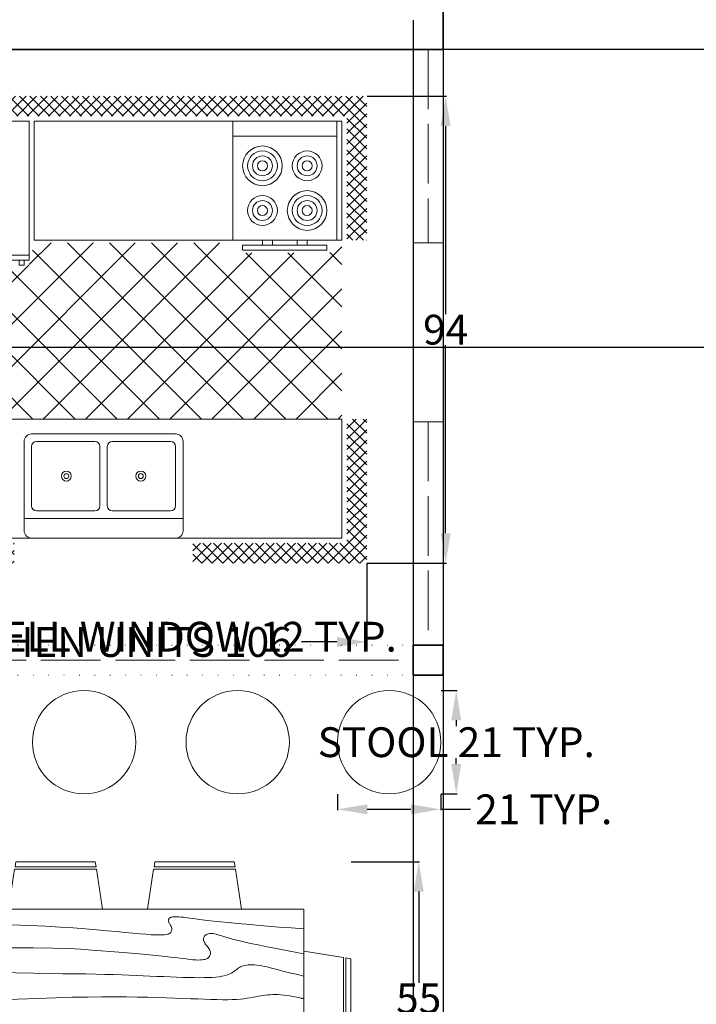
# Model space of a CAD drawing. Units: inches. Extents: x 823 to 1335, y 207 to 1074.
# Tile 4 of 6: x 943 to 1079, y 577 to 776. Entities that reach past the tile are written whole.
import ezdxf

# ---------------------------------------------------------------- set-up
doc = ezdxf.new("R2010")
doc.units = ezdxf.units.IN
doc.header["$MEASUREMENT"] = 0
doc.linetypes.add('ACAD_ISO02W100', pattern=[15, 12, -3])
doc.linetypes.add('ACAD_ISO07W100', pattern=[3, 0, -3])
for name, color, linetype, lineweight in [('A-ANNO-DIMS', 2, 'Continuous', 18), ('A-GLAZ-HIDN', 211, 'ACAD_ISO02W100', 18), ('A-GLAZ-OVHD', 211, 'ACAD_ISO07W100', 18), ('furniture', 21, 'Continuous', 18), ('inner wall', 102, 'Continuous', 35), ('kitchen', 171, 'Continuous', 18), ('windows', 211, 'Continuous', 18)]:
    doc.layers.add(name, color=color, linetype=linetype, lineweight=lineweight)
doc.styles.get("Standard").update_dxf_attribs({"font": 'arial.ttf'})
doc.dimstyles.get("Standard").update_dxf_attribs({"dimtxt": 6, "dimasz": 6, "dimexe": 0.18, "dimexo": 0.0625, "dimgap": 0.09, "dimtad": 0, "dimtih": 1, "dimtoh": 1, "dimdec": 0, "dimzin": 0, "dimdsep": 46, "dimlunit": 3, "dimtxsty": 'Standard', "dimcen": 0.09, "dimadec": 0, "dimazin": 0, "dimtfac": 1, "dimtdec": 0, "dimtofl": 0, "dimtmove": 0, "dimatfit": 3, "dimfxl": 1, "dimtolj": 1, "dimtzin": 0, "dimarcsym": 0})

# ---------------------------------------------------------------- blocks, each defined once
blk = doc.blocks.new('Dining Set - 36 x 72 in.')
for p, q in [((-22.2343, 26.00059), (-23.4847, 17.99762)), ((-22.2304, 26), (-5.7608, 26)), ((-22, 27.5), (-22.1562, 26.50042)), ((-5.8416, 26.5), (-22.1534, 26.5)), ((-22, 27.5), (-6, 27.5)), ((-5.8437, 26.49966), (-6, 27.5)), ((-4.5152, 17.99762), (-5.7655, 25.99926)), ((5.7657, 26.00059), (4.5153, 17.99762)), ((5.7696, 26), (22.2392, 26)), ((6, 27.5), (5.8438, 26.50042)), ((22.1584, 26.5), (5.8466, 26.5)), ((6, 27.5), (22, 27.5)), ((22.1563, 26.49966), (22, 27.5)), ((23.4848, 17.99762), (22.2345, 25.99926)), ((36, 18), (-36, 18)), ((-36, 18), (-36, -18)), ((36, -18), (36, 18)), ((-45.5, 8), (-44.5004, 8.15617)), ((-45.5, 8), (-45.5, -8)), ((-44.5, -8.15843), (-44.5, 8.15338)), ((-44.0006, 8.23428), (-35.9976, 9.48474)), ((-44, 8.23041), (-44, -8.23915)), ((44.0006, 8.23428), (35.9976, 9.48474)), ((44, 8.23041), (44, -8.23915)), ((44.5, -8.15843), (44.5, 8.15338)), ((45.5, 8), (44.5005, 8.15617)), ((45.5, 8), (45.5, -8)), ((-44.4997, -8.15631), (-45.5, -8)), ((-35.9976, -9.48476), (-43.9993, -8.2345)), ((35.9976, -9.48476), (43.9993, -8.2345)), ((44.4997, -8.15631), (45.5, -8)), ((-36, -18), (36, -18)), ((-22.2343, -26.0006), (-23.4847, -17.99762)), ((-4.5152, -17.99762), (-5.7655, -25.99928)), ((5.7657, -26.0006), (4.5153, -17.99762)), ((23.4848, -17.99762), (22.2345, -25.99928)), ((-22.2304, -26), (-5.7608, -26)), ((-22, -27.5), (-22.1562, -26.50044)), ((-5.8416, -26.5), (-22.1534, -26.5)), ((-22, -27.5), (-6, -27.5)), ((-5.8437, -26.49967), (-6, -27.5)), ((5.7696, -26), (22.2392, -26)), ((6, -27.5), (5.8438, -26.50044)), ((22.1584, -26.5), (5.8466, -26.5)), ((6, -27.5), (22, -27.5)), ((22.1563, -26.49967), (22, -27.5))]:
    blk.add_line(p, q)
for points in [[(-36, 15), (-31.1772, 14.97754), (-26.8079, 14.91406), (-22.8538, 14.81543), (-19.276, 14.6875), (-16.0362, 14.53613), (-13.0957, 14.36718), (-10.4159, 14.18652), (-7.9583, 14), (-5.6904, 13.81315), (-3.6035, 13.63021), (-1.6954, 13.45508), (0.0365, 13.29166), (1.5945, 13.14388), (2.9811, 13.01562), (4.1988, 12.9108), (5.25, 12.83333), (6.1393, 12.78613), (6.8802, 12.76823), (7.4883, 12.77767), (7.9792, 12.8125), (8.3685, 12.87077), (8.6719, 12.95052), (8.9049, 13.0498), (9.0833, 13.16666), (9.2205, 13.29899), (9.3216, 13.44401), (9.3895, 13.59879), (9.4271, 13.76041), (9.4373, 13.92594), (9.4232, 14.09245), (9.3875, 14.257), (9.3333, 14.41666), (9.2638, 14.56917), (9.1836, 14.71484), (9.0975, 14.85465), (9.0104, 14.98958), (8.9272, 15.1206), (8.8529, 15.2487), (8.7922, 15.37483), (8.75, 15.5), (8.7305, 15.62467), (8.7344, 15.74739), (8.7617, 15.86621), (8.8125, 15.97916), (8.8867, 16.08431), (8.9844, 16.17968), (9.1055, 16.26334), (9.25, 16.33333), (9.4189, 16.38802), (9.6172, 16.42708), (9.8506, 16.45052), (10.125, 16.45833), (10.4463, 16.45052), (10.8203, 16.42708), (11.2529, 16.38802), (11.75, 16.33333), (12.3184, 16.26318), (12.9694, 16.17838), (13.7151, 16.07991), (14.5677, 15.96875), (15.5395, 15.84586), (16.6426, 15.71224), (17.8893, 15.56884), (19.2917, 15.41666), (20.859, 15.25667), (22.5879, 15.08984), (24.4721, 14.91715), (26.5052, 14.73958), (28.6809, 14.5581), (30.9929, 14.3737), (33.4347, 14.18733), (36, 14)], [(-36, 10), (-28.9766, 10.14274), (-23.1725, 10.20442), (-18.4241, 10.19775), (-14.5677, 10.13541), (-11.4399, 10.03011), (-8.877, 9.89453), (-6.7154, 9.74137), (-4.7917, 9.58333), (-2.9698, 9.43082), (-1.2246, 9.28515), (0.4415, 9.14534), (2.026, 9.01041), (3.5266, 8.87939), (4.9408, 8.7513), (6.266, 8.62516), (7.5, 8.5), (8.6411, 8.37549), (9.6914, 8.2539), (10.6538, 8.13818), (11.5312, 8.03125), (12.3267, 7.93603), (13.043, 7.85547), (13.6831, 7.79248), (14.25, 7.75), (14.7471, 7.7303), (15.1797, 7.73307), (15.5537, 7.75732), (15.875, 7.80208), (16.1494, 7.86637), (16.3828, 7.94922), (16.5811, 8.04964), (16.75, 8.16666), (16.8944, 8.29915), (17.0143, 8.44531), (17.1089, 8.60319), (17.1771, 8.77083), (17.218, 8.94629), (17.2305, 9.1276), (17.2137, 9.31282), (17.1667, 9.5), (17.0895, 9.6875), (16.987, 9.875), (16.8649, 10.0625), (16.7292, 10.25), (16.5856, 10.4375), (16.4401, 10.625), (16.2985, 10.8125), (16.1667, 11), (16.05, 11.18733), (15.9518, 11.3737), (15.8752, 11.5581), (15.8229, 11.73958), (15.798, 11.91715), (15.8034, 12.08984), (15.842, 12.25667), (15.9167, 12.41666), (16.0295, 12.56836), (16.1784, 12.70833), (16.3605, 12.83268), (16.5729, 12.9375), (16.8127, 13.01888), (17.0768, 13.07291), (17.3625, 13.0957), (17.6667, 13.08333), (17.9894, 13.03312), (18.3418, 12.94726), (18.7382, 12.82918), (19.1927, 12.68229), (19.7195, 12.51001), (20.3327, 12.31575), (21.0465, 12.10294), (21.875, 11.875), (22.8357, 11.63354), (23.959, 11.37304), (25.2786, 11.08618), (26.8282, 10.76562), (28.6414, 10.40405), (30.752, 9.99414), (33.1936, 9.52856), (36, 9)], [(-36, 5.5), (-30.7157, 5.3348), (-26.069, 5.20963), (-21.9946, 5.11767), (-18.4271, 5.05208), (-15.3009, 5.00602), (-12.5508, 4.97265), (-10.1112, 4.94515), (-7.9167, 4.91666), (-5.909, 4.88167), (-4.0586, 4.83984), (-2.3429, 4.79215), (-0.7396, 4.73958), (0.7739, 4.6831), (2.22, 4.6237), (3.6213, 4.56233), (5, 4.5), (6.373, 4.43782), (7.7344, 4.3776), (9.0723, 4.32129), (10.375, 4.27083), (11.6309, 4.22819), (12.8281, 4.19531), (13.9551, 4.17415), (15, 4.16666), (15.954, 4.17448), (16.819, 4.19791), (17.6001, 4.23698), (18.3021, 4.29166), (18.9299, 4.36198), (19.4883, 4.44791), (19.9823, 4.54948), (20.4167, 4.66666), (20.7969, 4.79899), (21.1302, 4.94401), (21.4245, 5.09879), (21.6875, 5.26041), (21.9271, 5.42594), (22.1511, 5.59245), (22.3672, 5.757), (22.5834, 5.91666), (22.8065, 6.06868), (23.0404, 6.21093), (23.2879, 6.34147), (23.5521, 6.45833), (23.8358, 6.55957), (24.142, 6.64323), (24.4735, 6.70735), (24.8334, 6.75), (25.2235, 6.76969), (25.642, 6.76692), (26.0858, 6.74267), (26.5521, 6.69791), (27.0379, 6.63362), (27.5404, 6.55078), (28.0565, 6.45036), (28.5834, 6.33333), (29.1242, 6.19987), (29.7071, 6.04687), (30.3661, 5.87044), (31.1354, 5.66666), (32.0493, 5.43164), (33.142, 5.16146), (34.4475, 4.85221), (36, 4.5)], [(-36, -1), (-30.7915, -0.6591), (-26.0195, -0.38216), (-21.6519, -0.16284), (-17.6563, 0.00521), (-14.0005, 0.12833), (-10.6523, 0.21289), (-7.5796, 0.26522), (-4.75, 0.29166), (-2.134, 0.29793), (0.2878, 0.28711), (2.5317, 0.26163), (4.6146, 0.22396), (6.5529, 0.17651), (8.3633, 0.12174), (10.0623, 0.06209), (11.6667, 0), (13.1899, -0.06201), (14.6341, -0.1211), (15.9982, -0.17432), (17.2813, -0.21875), (18.4823, -0.25147), (19.6003, -0.26953), (20.6343, -0.27002), (21.5834, -0.25), (22.4481, -0.20768), (23.2357, -0.14584), (23.9549, -0.06836), (24.6146, 0.02083), (25.2235, 0.11784), (25.7904, 0.21875), (26.3241, 0.31966), (26.8334, 0.41666), (27.3265, 0.50618), (27.8099, 0.58593), (28.2894, 0.65397), (28.7709, 0.70833), (29.2601, 0.74707), (29.763, 0.76823), (30.2855, 0.76985), (30.8334, 0.75), (31.4088, 0.70784), (31.9994, 0.64713), (32.589, 0.57275), (33.1615, 0.48958), (33.7008, 0.4025), (34.1908, 0.3164), (34.6153, 0.23616), (34.9584, 0.16666), (35.2099, 0.11165), (35.3848, 0.07031), (35.504, 0.04069), (35.5886, 0.02083), (35.6594, 0.00879), (35.7377, 0.0026), (35.8442, 0.00032), (36, 0)], [(-36, -6.5), (-27.1843, -6.31267), (-20.084, -6.1263), (-14.469, -5.9419), (-10.1094, -5.76042), (-6.7752, -5.58285), (-4.2363, -5.41016), (-2.2629, -5.24333), (-0.625, -5.08334), (0.8708, -4.93099), (2.2715, -4.78646), (3.5872, -4.64974), (4.8281, -4.52084), (6.0046, -4.39974), (7.127, -4.28646), (8.2053, -4.18099), (9.25, -4.08334), (10.2705, -3.99382), (11.2734, -3.91407), (12.2647, -3.84603), (13.25, -3.79167), (14.2354, -3.75293), (15.2266, -3.73177), (16.2295, -3.73015), (17.25, -3.75), (18.2912, -3.79248), (19.3451, -3.85547), (20.4009, -3.93604), (21.4479, -4.03125), (22.4754, -4.13819), (23.4727, -4.25391), (24.4289, -4.37549), (25.3334, -4.5), (26.1785, -4.62492), (26.9694, -4.74935), (27.7145, -4.87281), (28.4219, -4.99479), (29.1, -5.11483), (29.7572, -5.23242), (30.4016, -5.34709), (31.0417, -5.45834), (31.6837, -5.56437), (32.3262, -5.65821), (32.9658, -5.73153), (33.599, -5.77604), (34.2224, -5.78345), (34.8327, -5.74545), (35.4264, -5.65373), (36, -5.5)], [(-36, -10), (-26.4022, -9.81299), (-18.4675, -9.62891), (-11.9839, -9.45069), (-6.7396, -9.28125), (-2.5226, -9.12354), (0.8789, -8.98047), (3.6769, -8.85498), (6.0833, -8.75), (8.2767, -8.66765), (10.3021, -8.60677), (12.1712, -8.56543), (13.8958, -8.54167), (15.4876, -8.53353), (16.9583, -8.53907), (18.3197, -8.55632), (19.5834, -8.58334), (20.7616, -8.61841), (21.8685, -8.66081), (22.9188, -8.71004), (23.9271, -8.76563), (24.9081, -8.82707), (25.8763, -8.89388), (26.8465, -8.96558), (27.8334, -9.04167), (28.8474, -9.12118), (29.8828, -9.20117), (30.93, -9.27824), (31.9792, -9.34896), (33.0205, -9.40991), (34.0443, -9.45768), (35.0407, -9.48885), (36, -9.5)], [(-36, -14.5), (-30.0881, -14.33513), (-25.0332, -14.21224), (-20.7312, -14.12647), (-17.0781, -14.07292), (-13.97, -14.04671), (-11.3027, -14.04297), (-8.9724, -14.05681), (-6.875, -14.08334), (-4.9224, -14.11833), (-3.0905, -14.16016), (-1.3709, -14.20785), (0.2448, -14.26042), (1.7647, -14.3169), (3.1973, -14.3763), (4.5507, -14.43767), (5.8333, -14.5), (7.0554, -14.5621), (8.235, -14.62175), (9.3922, -14.67652), (10.5469, -14.72396), (11.7192, -14.76164), (12.929, -14.78711), (14.1965, -14.79794), (15.5417, -14.79167), (16.9933, -14.76424), (18.6152, -14.70508), (20.4804, -14.60197), (22.6615, -14.44271), (25.2312, -14.21509), (28.2624, -13.9069), (31.8277, -13.50594), (36, -13)]]:
    blk.add_lwpolyline(points)
blk = doc.blocks.new('Kitchen Layout - 7 x 8 ft')
for p, q in [((-5, 81.32), (2.68, 89)), ((-5, 83.44), (0.56, 89)), ((-5, 85.56), (-1.56, 89)), ((-5, 87.68), (-3.68, 89)), ((-1, 84.97), (-5, 88.97)), ((1.09, 85), (-2.91, 89)), ((3.21, 85), (-0.79, 89)), ((0.81, 85), (4.81, 89)), ((5.34, 85), (1.34, 89)), ((2.93, 85), (6.93, 89)), ((7.46, 85), (3.46, 89)), ((5.05, 85), (9.05, 89)), ((9.58, 85), (5.58, 89)), ((7.17, 85), (11.17, 89)), ((11.7, 85), (7.7, 89)), ((9.29, 85), (13.29, 89)), ((13.82, 85), (9.82, 89)), ((11.41, 85), (15.41, 89)), ((15.94, 85), (11.94, 89)), ((13.53, 85), (17.53, 89)), ((18.06, 85), (14.06, 89)), ((15.65, 85), (19.65, 89)), ((20.18, 85), (16.18, 89)), ((17.78, 85), (21.78, 89)), ((22.31, 85), (18.31, 89)), ((19.9, 85), (23.9, 89)), ((24.43, 85), (20.43, 89)), ((22.02, 85), (26.02, 89)), ((26.55, 85), (22.55, 89)), ((24.14, 85), (28.14, 89)), ((28.67, 85), (24.67, 89)), ((26.26, 85), (30.26, 89)), ((30.79, 85), (26.79, 89)), ((28.38, 85), (32.38, 89)), ((32.91, 85), (28.91, 89)), ((30.5, 85), (34.5, 89)), ((35.03, 85), (31.03, 89)), ((32.63, 85), (36.63, 89)), ((37.16, 85), (33.16, 89)), ((34.75, 85), (38.75, 89)), ((39.28, 85), (35.28, 89)), ((36.87, 85), (40.87, 89)), ((41.4, 85), (37.4, 89)), ((38.99, 85), (42.99, 89)), ((43.52, 85), (39.52, 89)), ((41.11, 85), (45.11, 89)), ((45.64, 85), (41.64, 89)), ((43.23, 85), (47.23, 89)), ((47.76, 85), (43.76, 89)), ((45.35, 85), (49.35, 89)), ((49.88, 85), (45.88, 89)), ((47.47, 85), (51.47, 89)), ((52, 85), (48, 89)), ((49.6, 85), (53.6, 89)), ((54.13, 85), (50.13, 89)), ((51.72, 85), (55.72, 89)), ((56.25, 85), (52.25, 89)), ((53.84, 85), (57.84, 89)), ((58.37, 85), (54.37, 89)), ((55.96, 85), (59.96, 89)), ((60.49, 85), (56.49, 89)), ((58.08, 85), (62.08, 89)), ((62.61, 85), (58.61, 89)), ((60.2, 85), (64.2, 89)), ((64.73, 85), (60.73, 89)), ((62.32, 85), (66.32, 89)), ((66.85, 85), (62.85, 89)), ((64.45, 85), (68.45, 89)), ((68.97, 85), (64.97, 89)), ((66.57, 85), (70.57, 89)), ((71.1, 85), (67.1, 89)), ((68.69, 85), (72.69, 89)), ((73.22, 85), (69.22, 89)), ((70.81, 85), (74.81, 89)), ((75.34, 85), (71.34, 89)), ((72.93, 85), (76.93, 89)), ((77.46, 85), (73.46, 89)), ((75.05, 85), (79.05, 89)), ((79.58, 85), (75.58, 89)), ((77.17, 85), (81.17, 89)), ((81.7, 85), (77.7, 89)), ((79.29, 85), (83.29, 89)), ((83.82, 85), (79.82, 89)), ((81.42, 85), (85.42, 89)), ((85.95, 85), (81.95, 89)), ((83.54, 85), (87.54, 89)), ((88.07, 85), (84.07, 89)), ((85.66, 85), (89.66, 89)), ((90.19, 85), (86.19, 89)), ((87.78, 85), (91.78, 89)), ((92.31, 85), (88.31, 89)), ((89.9, 85), (93.9, 89)), ((94.43, 85), (90.43, 89)), ((92.02, 85), (96.02, 89)), ((96.55, 85), (92.55, 89)), ((94.14, 85), (98.14, 89)), ((101, 82.67), (94.67, 89)), ((96.27, 85), (100.27, 89)), ((101, 84.79), (96.79, 89)), ((97, 83.61), (101, 87.61)), ((101, 86.92), (98.92, 89)), ((-1, 82.85), (-5, 86.85)), ((97, 81.49), (101, 85.49)), ((-1, 80.73), (-5, 84.73)), ((34, 84), (96, 84)), ((34, 60), (34, 84)), ((96, 84), (96, 60)), ((101, 80.55), (97, 84.55)), ((97, 79.37), (101, 83.37)), ((-5, 79.19), (-1, 83.19)), ((-1, 78.61), (-5, 82.61)), ((101, 78.43), (97, 82.43)), ((-5, 77.07), (-1, 81.07)), ((-1, 76.49), (-5, 80.49)), ((74, 81), (95, 81)), ((97, 77.25), (101, 81.25)), ((101, 76.31), (97, 80.31)), ((-5, 74.95), (-1, 78.95)), ((-1, 74.36), (-5, 78.36)), ((97, 75.13), (101, 79.13)), ((101, 74.19), (97, 78.19)), ((-5, 72.83), (-1, 76.83)), ((-1, 72.24), (-5, 76.24)), ((97, 73.01), (101, 77.01)), ((101, 72.07), (97, 76.07)), ((-5, 70.71), (-1, 74.71)), ((-1, 70.12), (-5, 74.12)), ((97, 70.89), (101, 74.89)), ((101, 69.95), (97, 73.95)), ((-5, 68.59), (-1, 72.59)), ((-1, 68), (-5, 72)), ((97, 68.76), (101, 72.76)), ((101, 67.82), (97, 71.82)), ((-5, 66.47), (-1, 70.47)), ((-1, 65.88), (-5, 69.88)), ((97, 66.64), (101, 70.64)), ((101, 65.7), (97, 69.7)), ((-5, 64.35), (-1, 68.35)), ((-1, 63.76), (-5, 67.76)), ((97, 64.52), (101, 68.52)), ((101, 63.58), (97, 67.58)), ((-5, 62.22), (-1, 66.22)), ((-1, 61.64), (-5, 65.64)), ((97, 62.4), (101, 66.4)), ((101, 61.46), (97, 65.46)), ((-5, 60.1), (-1, 64.1)), ((-1, 59.52), (-5, 63.52)), ((97, 60.28), (101, 64.28)), ((-5, 57.98), (-1, 61.98)), ((100.34, 60), (97, 63.34)), ((98.84, 60), (101, 62.16)), ((-1, 57.39), (-5, 61.39)), ((-4.86, 56), (-1, 59.86)), ((10.4, 24), (45.9, 59.5)), ((18.88, 24), (54.38, 59.5)), ((27.37, 24), (62.87, 59.5)), ((33.03, 55.11), (37.41, 59.5)), ((96, 60), (34, 60)), ((35.85, 24), (71.35, 59.5)), ((76.2, 24), (40.7, 59.5)), ((84.68, 24), (49.18, 59.5)), ((93.17, 24), (57.67, 59.5)), ((96, 29.65), (66.15, 59.5)), ((80, 60), (80, 59)), ((82, 59), (82, 60)), ((87, 59), (87, 60)), ((89, 60), (89, 59)), ((98.22, 60), (97, 61.22)), ((100.96, 60), (101, 60.04)), ((-1.73, 56), (-5, 59.27)), ((-2.74, 56), (-1, 57.74)), ((67.71, 24), (33.68, 58.04)), ((61.31, 24), (96, 58.69)), ((96, 55.11), (93.57, 57.54)), ((-3.85, 56), (-5, 57.15)), ((0, 57), (33, 57)), ((31, 55), (31, 56)), ((32, 56), (32, 55)), ((44.34, 24), (77.84, 57.5)), ((52.82, 24), (86.32, 57.5)), ((96, 38.14), (76.64, 57.5)), ((96, 46.63), (85.13, 57.5)), ((0, 30.57), (24.43, 55)), ((0, 39.06), (15.94, 55)), ((0, 47.54), (7.46, 55)), ((1.91, 24), (32.91, 55)), ((33.77, 24), (2.77, 55)), ((42.26, 24), (11.26, 55)), ((50.74, 24), (19.74, 55)), ((59.23, 24), (28.23, 55)), ((32, 55), (31, 55)), ((69.79, 24), (96, 50.21)), ((25.29, 24), (0, 49.29)), ((78.28, 24), (96, 41.72)), ((16.8, 24), (0, 40.8)), ((8.32, 24), (0, 32.32)), ((86.76, 24), (96, 33.24)), ((-5, 21.92), (-2.92, 24)), ((-1, 21.33), (-3.67, 24)), ((-1, 23.45), (-1.55, 24)), ((0, 24), (96, 24)), ((0, 0), (0, 24)), ((95.25, 24), (96, 24.75)), ((96, 24), (96, 0)), ((97, 22.1), (98.9, 24)), ((97, 19.97), (101, 23.97)), ((101, 21.16), (98.16, 24)), ((101, 23.28), (100.28, 24)), ((-5, 19.8), (-1, 23.8)), ((-1, 19.21), (-5, 23.21)), ((101, 19.03), (97, 23.03)), ((97, 17.85), (101, 21.85)), ((-5, 17.68), (-1, 21.68)), ((-1, 17.09), (-5, 21.09)), ((101, 16.91), (97, 20.91)), ((-5, 15.55), (-1, 19.55)), ((-1, 14.97), (-5, 18.97)), ((47.25, 6.5), (47.25, 18.5)), ((48.75, 18.5), (48.75, 6.5)), ((97, 15.73), (101, 19.73)), ((101, 14.79), (97, 18.79)), ((-5, 13.43), (-1, 17.43)), ((-1, 12.85), (-5, 16.85)), ((97, 13.61), (101, 17.61)), ((101, 12.67), (97, 16.67)), ((-5, 11.31), (-1, 15.31)), ((-1, 10.73), (-5, 14.73)), ((97, 11.49), (101, 15.49)), ((101, 10.55), (97, 14.55)), ((-5, 9.19), (-1, 13.19)), ((-1, 8.6), (-5, 12.6)), ((97, 9.37), (101, 13.37)), ((101, 8.43), (97, 12.43)), ((-5, 7.07), (-1, 11.07)), ((-1, 6.48), (-5, 10.48)), ((97, 7.25), (101, 11.25)), ((101, 6.31), (97, 10.31)), ((-5, 4.95), (-1, 8.95)), ((-1, 4.36), (-5, 8.36)), ((97, 5.12), (101, 9.12)), ((101, 4.18), (97, 8.18)), ((-5, 2.83), (-1, 6.83)), ((-1, 2.24), (-5, 6.24)), ((97, 3), (101, 7)), ((101, 2.06), (97, 6.06)), ((-5, 0.71), (-1, 4.71)), ((-1, 0.12), (-5, 4.12)), ((64, 4), (32, 4)), ((97, 0.88), (101, 4.88)), ((-5, -1.42), (-1, 2.58)), ((2, -5), (-5, 2)), ((93.24, -5), (101, 2.76)), ((101, -0.06), (97, 3.94)), ((-5, -3.54), (-1, 0.46)), ((96, 0), (0, 0)), ((95.36, -5), (101, 0.64)), ((101, -2.18), (97, 1.82)), ((-0.12, -5), (-5, -0.12)), ((-4.34, -5), (-0.34, -1)), ((-2.22, -5), (1.78, -1)), ((-0.1, -5), (3.9, -1)), ((4.12, -5), (0.12, -1)), ((2.02, -5), (6.02, -1)), ((6.24, -5), (2.24, -1)), ((4.14, -5), (8.14, -1)), ((8.36, -5), (4.36, -1)), ((6.27, -5), (10.27, -1)), ((10.48, -5), (6.48, -1)), ((8.39, -5), (12.39, -1)), ((12.6, -5), (8.6, -1)), ((10.51, -5), (14.51, -1)), ((14.73, -5), (10.73, -1)), ((12.63, -5), (16.63, -1)), ((16.85, -5), (12.85, -1)), ((14.75, -5), (18.75, -1)), ((18.97, -5), (14.97, -1)), ((16.87, -5), (20.87, -1)), ((21.09, -5), (17.09, -1)), ((18.99, -5), (22.99, -1)), ((23.21, -5), (19.21, -1)), ((21.11, -5), (25.11, -1)), ((25.33, -5), (21.33, -1)), ((23.24, -5), (27.24, -1)), ((27.45, -5), (23.45, -1)), ((25.36, -5), (29.36, -1)), ((29.57, -5), (25.57, -1)), ((30, -3.3), (27.7, -1)), ((30, -1.18), (29.82, -1)), ((66, -2.54), (67.54, -1)), ((66, -4.66), (69.66, -1)), ((69.88, -5), (66, -1.12)), ((67.78, -5), (71.78, -1)), ((72, -5), (68, -1)), ((69.9, -5), (73.9, -1)), ((74.12, -5), (70.12, -1)), ((72.03, -5), (76.03, -1)), ((76.24, -5), (72.24, -1)), ((74.15, -5), (78.15, -1)), ((78.36, -5), (74.36, -1)), ((76.27, -5), (80.27, -1)), ((80.49, -5), (76.49, -1)), ((78.39, -5), (82.39, -1)), ((82.61, -5), (78.61, -1)), ((80.51, -5), (84.51, -1)), ((84.73, -5), (80.73, -1)), ((82.63, -5), (86.63, -1)), ((86.85, -5), (82.85, -1)), ((84.75, -5), (88.75, -1)), ((88.97, -5), (84.97, -1)), ((86.88, -5), (90.88, -1)), ((91.09, -5), (87.09, -1)), ((89, -5), (93, -1)), ((93.21, -5), (89.21, -1)), ((91.12, -5), (95.12, -1)), ((95.34, -5), (91.34, -1)), ((97.46, -5), (93.46, -1)), ((99.58, -5), (95.58, -1)), ((101, -4.3), (97, -0.3)), ((97.48, -5), (101, -1.48)), ((-2.25, -5), (-5, -2.25)), ((27.48, -5), (30, -2.48)), ((67.76, -5), (66, -3.24)), ((99.6, -5), (101, -3.6)), ((-4.37, -5), (-5, -4.37)), ((29.6, -5), (30, -4.6))]:
    blk.add_line(p, q)
for points in [[(0, 56), (0, 84), (33, 84), (33, 56)], [(74, 60), (74, 84), (95, 84), (95, 60)], [(76, 58), (76, 59), (93, 59), (93, 58)]]:
    blk.add_lwpolyline(points, close=True)
for points in [[(33.5, 21), (62.5, 21)], [(32, 1.5), (32, 19.5)], [(33.5, 6.5), (33.5, 18.5)], [(34.5, 19.5), (46.25, 19.5)], [(49.75, 19.5), (61.5, 19.5)], [(62.5, 18.5), (62.5, 6.5)], [(64, 19.5), (64, 1.5)], [(46.25, 5.5), (34.5, 5.5)], [(61.5, 5.5), (49.75, 5.5)], [(62.5, 0), (33.5, 0)]]:
    blk.add_lwpolyline(points)
for centre, radius in [((80, 75), 4), ((80, 75), 3), ((89, 75), 3), ((80, 75), 2), ((80, 75), 1), ((89, 75), 2), ((89, 75), 1), ((89, 66), 4), ((80, 66), 3), ((80, 66), 2), ((89, 66), 3), ((89, 66), 2), ((80, 66), 1), ((89, 66), 1), ((40.5, 12.5), 1), ((40.5, 12.5), 0.5), ((55.5, 12.5), 1), ((55.5, 12.5), 0.5)]:
    blk.add_circle(centre, radius)
for centre, radius, start, end in [((33.5, 19.5), 1.5, 90, 180), ((62.5, 19.5), 1.5, 0, 90), ((34.5, 18.5), 1, 90, 180), ((46.25, 18.5), 1, 0, 90), ((49.75, 18.5), 1, 90, 180), ((61.5, 18.5), 1, 0, 90), ((34.5, 6.5), 1, 180, 270), ((46.25, 6.5), 1, 270, 0), ((49.75, 6.5), 1, 180, 270), ((61.5, 6.5), 1, 270, 0), ((33.5, 1.5), 1.5, 180, 270), ((62.5, 1.5), 1.5, 270, 0)]:
    blk.add_arc(centre, radius, start, end)
blk = doc.blocks.new('STOOL-COUNTER-ROUND')
blk.add_circle((10.41, 10.41), 10.41)
blk = doc.blocks.new('*D31')
at = {"layer": 'A-ANNO-DIMS', "color": 0, "lineweight": -2, "transparency": 16777216}
for p, q in [((1009.76, 605.98), (1023.52, 605.98)), ((1023.34, 599.98), (1023.34, 581.62)), ((1023.34, 556.98), (1023.34, 575.34)), ((1009.76, 550.98), (1023.52, 550.98))]:
    blk.add_line(p, q, dxfattribs=at)
for points in [[(1022.34, 599.98), (1024.34, 599.98), (1023.34, 605.98)], [(1022.34, 556.98), (1024.34, 556.98), (1023.34, 550.98)]]:
    blk.add_solid(points, dxfattribs=at)
at = {"layer": 'Defpoints', "color": 0, "lineweight": -2, "transparency": 16777216}
for p in [(1009.69, 605.98), (1023.34, 605.98), (1009.69, 550.98)]:
    blk.add_point(p, dxfattribs=at)
at = {"layer": 'A-ANNO-DIMS', "color": 0, "transparency": 16777216, "insert": (1023.34, 578.48), "char_height": 6, "attachment_point": 5}
blk.add_mtext('\\A1;55', dxfattribs=at)
blk = doc.blocks.new('*D32')
at = {"layer": 'A-ANNO-DIMS', "color": 0, "lineweight": -2, "transparency": 16777216}
for p, q in [((906.87, 666.11), (906.87, 650.09)), ((1012.87, 666.11), (1012.87, 650.09)), ((912.87, 650.27), (919.99, 650.27)), ((1006.87, 650.27), (999.75, 650.27))]:
    blk.add_line(p, q, dxfattribs=at)
for points in [[(912.87, 651.27), (912.87, 649.27), (906.87, 650.27)], [(1006.87, 651.27), (1006.87, 649.27), (1012.87, 650.27)]]:
    blk.add_solid(points, dxfattribs=at)
at = {"layer": 'Defpoints', "color": 0, "lineweight": -2, "transparency": 16777216}
for p in [(906.87, 666.17), (1012.87, 666.17), (1012.87, 650.27)]:
    blk.add_point(p, dxfattribs=at)
at = {"layer": 'A-ANNO-DIMS', "color": 0, "transparency": 16777216, "insert": (959.87, 650.27), "char_height": 6, "attachment_point": 5}
blk.add_mtext('\\A1;KITCHEN UNITS 106', dxfattribs=at)
blk = doc.blocks.new('*D33')
at = {"layer": 'A-ANNO-DIMS', "color": 0, "lineweight": -2, "transparency": 16777216}
for p, q in [((1012.93, 760.17), (1028.95, 760.17)), ((1028.77, 754.17), (1028.77, 716.32)), ((1028.77, 672.17), (1028.77, 710.02)), ((1012.93, 666.17), (1028.95, 666.17))]:
    blk.add_line(p, q, dxfattribs=at)
for points in [[(1027.77, 754.17), (1029.77, 754.17), (1028.77, 760.17)], [(1027.77, 672.17), (1029.77, 672.17), (1028.77, 666.17)]]:
    blk.add_solid(points, dxfattribs=at)
at = {"layer": 'Defpoints', "color": 0, "lineweight": -2, "transparency": 16777216}
for p in [(1012.87, 760.17), (1028.77, 760.17), (1012.87, 666.17)]:
    blk.add_point(p, dxfattribs=at)
at = {"layer": 'A-ANNO-DIMS', "color": 0, "transparency": 16777216, "insert": (1028.77, 713.17), "char_height": 6, "attachment_point": 5}
blk.add_mtext('\\A1;94', dxfattribs=at)
blk = doc.blocks.new('*D36')
at = {"layer": 'A-ANNO-DIMS', "color": 0, "lineweight": -2, "transparency": 16777216}
for p, q in [((1027.85, 640.49), (1031.09, 640.49)), ((1030.91, 634.49), (1030.91, 633.28)), ((1030.91, 625.68), (1030.91, 626.89)), ((1027.85, 619.68), (1031.09, 619.68))]:
    blk.add_line(p, q, dxfattribs=at)
for points in [[(1029.91, 634.49), (1031.91, 634.49), (1030.91, 640.49)], [(1029.91, 625.68), (1031.91, 625.68), (1030.91, 619.68)]]:
    blk.add_solid(points, dxfattribs=at)
at = {"layer": 'Defpoints', "color": 0, "lineweight": -2, "transparency": 16777216}
for p in [(1027.79, 640.49), (1030.91, 640.49), (1027.79, 619.68)]:
    blk.add_point(p, dxfattribs=at)
at = {"layer": 'A-ANNO-DIMS', "color": 0, "transparency": 16777216, "insert": (1030.91, 630.08), "char_height": 6, "attachment_point": 5}
blk.add_mtext('\\A1;STOOL 21 TYP.', dxfattribs=at)
blk = doc.blocks.new('*D37')
at = {"layer": 'A-ANNO-DIMS', "color": 0, "lineweight": -2, "transparency": 16777216}
for p, q in [((1006.97, 619.62), (1006.97, 616.38)), ((1027.79, 619.62), (1027.79, 616.38)), ((1012.97, 616.56), (1021.79, 616.56)), ((1027.79, 616.56), (1033.79, 616.56))]:
    blk.add_line(p, q, dxfattribs=at)
for points in [[(1012.97, 617.56), (1012.97, 615.56), (1006.97, 616.56)], [(1021.79, 617.56), (1021.79, 615.56), (1027.79, 616.56)]]:
    blk.add_solid(points, dxfattribs=at)
at = {"layer": 'Defpoints', "color": 0, "lineweight": -2, "transparency": 16777216}
for p in [(1006.97, 619.68), (1027.79, 619.68), (1027.79, 616.56)]:
    blk.add_point(p, dxfattribs=at)
at = {"layer": 'A-ANNO-DIMS', "color": 0, "transparency": 16777216, "insert": (1048.53, 616.56), "char_height": 6, "attachment_point": 5}
blk.add_mtext('\\A1;21 TYP.', dxfattribs=at)
blk = doc.blocks.new('*D50')
at = {"layer": 'A-ANNO-DIMS', "color": 0, "lineweight": -2, "transparency": 16777216}
for p, q in [((875.44, 651.33), (869.44, 651.33)), ((881.44, 649.67), (881.44, 651.51)), ((892.95, 649.67), (892.95, 651.51)), ((898.95, 651.33), (904.95, 651.33))]:
    blk.add_line(p, q, dxfattribs=at)
for points in [[(875.44, 652.33), (875.44, 650.33), (881.44, 651.33)], [(898.95, 652.33), (898.95, 650.33), (892.95, 651.33)]]:
    blk.add_solid(points, dxfattribs=at)
at = {"layer": 'Defpoints', "color": 0, "lineweight": -2, "transparency": 16777216}
for p in [(892.95, 651.33), (881.44, 649.61), (892.95, 649.61)]:
    blk.add_point(p, dxfattribs=at)
at = {"layer": 'A-ANNO-DIMS', "color": 0, "transparency": 16777216, "insert": (963.98, 651.33), "char_height": 6, "attachment_point": 5}
blk.add_mtext('\\A1;LIGHTWELL WINDOW 12 TYP.', dxfattribs=at)
blk = doc.blocks.new('*D60')
at = {"layer": 'A-ANNO-DIMS', "color": 0, "lineweight": -2, "transparency": 16777216}
for p, q in [((878.26, 775.54), (878.26, 211.18)), ((1022.26, 775.54), (1022.26, 211.18)), ((884.26, 211.36), (943.84, 211.36)), ((1016.26, 211.36), (956.69, 211.36))]:
    blk.add_line(p, q, dxfattribs=at)
for points in [[(884.26, 212.36), (884.26, 210.36), (878.26, 211.36)], [(1016.26, 212.36), (1016.26, 210.36), (1022.26, 211.36)]]:
    blk.add_solid(points, dxfattribs=at)
at = {"layer": 'Defpoints', "color": 0, "lineweight": -2, "transparency": 16777216}
for p in [(878.26, 775.61), (1022.26, 775.61), (1022.26, 211.36)]:
    blk.add_point(p, dxfattribs=at)
at = {"layer": 'A-ANNO-DIMS', "color": 0, "transparency": 16777216, "insert": (950.26, 211.36), "char_height": 6, "attachment_point": 5}
blk.add_mtext('\\A1;144', dxfattribs=at)
blk = doc.blocks.new('*D61')
at = {"layer": 'A-ANNO-DIMS', "color": 0, "lineweight": -2, "transparency": 16777216}
for p, q in [((1028.26, 847.54), (1028.26, 211.18)), ((1088.26, 847.54), (1088.26, 211.18)), ((1034.26, 211.36), (1053.87, 211.36)), ((1082.26, 211.36), (1062.66, 211.36))]:
    blk.add_line(p, q, dxfattribs=at)
for points in [[(1034.26, 212.36), (1034.26, 210.36), (1028.26, 211.36)], [(1082.26, 212.36), (1082.26, 210.36), (1088.26, 211.36)]]:
    blk.add_solid(points, dxfattribs=at)
at = {"layer": 'Defpoints', "color": 0, "lineweight": -2, "transparency": 16777216}
for p in [(1028.26, 847.61), (1088.26, 847.61), (1088.26, 211.36)]:
    blk.add_point(p, dxfattribs=at)
at = {"layer": 'A-ANNO-DIMS', "color": 0, "transparency": 16777216, "insert": (1058.26, 211.36), "char_height": 6, "attachment_point": 5}
blk.add_mtext('\\A1;60', dxfattribs=at)
blk = doc.blocks.new('*D66')
at = {"layer": 'A-ANNO-DIMS', "color": 0, "lineweight": -2, "transparency": 16777216}
for p, q in [((902.26, 769.67), (902.26, 1070.04)), ((908.26, 1069.86), (958.83, 1069.86)), ((1022.26, 1069.86), (971.7, 1069.86)), ((1028.26, 769.67), (1028.26, 1070.04))]:
    blk.add_line(p, q, dxfattribs=at)
for points in [[(908.26, 1070.86), (908.26, 1068.86), (902.26, 1069.86)], [(1022.26, 1070.86), (1022.26, 1068.86), (1028.26, 1069.86)]]:
    blk.add_solid(points, dxfattribs=at)
at = {"layer": 'Defpoints', "color": 0, "lineweight": -2, "transparency": 16777216}
for p in [(1028.26, 1069.86), (902.26, 769.61), (1028.26, 769.61)]:
    blk.add_point(p, dxfattribs=at)
at = {"layer": 'A-ANNO-DIMS', "color": 0, "transparency": 16777216, "insert": (965.26, 1069.86), "char_height": 6, "attachment_point": 5}
blk.add_mtext('\\A1;126', dxfattribs=at)
blk = doc.blocks.new('*D70')
at = {"layer": 'A-ANNO-DIMS', "color": 0, "lineweight": -2, "transparency": 16777216}
for p, q in [((1094.2, 769.61), (829.83, 769.61)), ((830.01, 763.61), (830.01, 742.76)), ((830.01, 715.61), (830.01, 736.45)), ((1094.2, 709.61), (829.83, 709.61))]:
    blk.add_line(p, q, dxfattribs=at)
for points in [[(829.01, 763.61), (831.01, 763.61), (830.01, 769.61)], [(829.01, 715.61), (831.01, 715.61), (830.01, 709.61)]]:
    blk.add_solid(points, dxfattribs=at)
at = {"layer": 'Defpoints', "color": 0, "lineweight": -2, "transparency": 16777216}
for p in [(1094.26, 769.61), (830.01, 709.61), (1094.26, 709.61)]:
    blk.add_point(p, dxfattribs=at)
at = {"layer": 'A-ANNO-DIMS', "color": 0, "transparency": 16777216, "insert": (830.01, 739.61), "char_height": 6, "attachment_point": 5}
blk.add_mtext('\\A1;60', dxfattribs=at)

msp = doc.modelspace()

# ---------------------------------------------------------------- linework, layer by layer
at = {"layer": 'A-GLAZ-HIDN'}
for p, q in [((1022.26, 769.61), (1028.26, 769.61)), ((1025.26, 769.61), (1025.26, 730.68)), ((1022.26, 730.68), (1028.26, 730.68)), ((1025.26, 694.64), (1025.26, 649.61)), ((902.26, 646.61), (1022.26, 646.61))]:
    msp.add_line(p, q, dxfattribs=at)
at = {"layer": 'A-GLAZ-OVHD'}
for p, q in [((1022.26, 769.61), (1022.26, 730.68)), ((1028.26, 769.61), (1028.26, 730.68)), ((1022.26, 694.64), (1022.26, 649.61)), ((1028.26, 694.64), (1028.26, 649.61)), ((902.26, 649.61), (1022.26, 649.61)), ((902.26, 643.61), (1022.26, 643.61))]:
    msp.add_line(p, q, dxfattribs=at)
at = {"layer": 'inner wall'}
for p, q in [((1028.26, 769.61), (1028.26, 779.51)), ((902.26, 769.61), (1028.26, 769.61)), ((1022.26, 649.61), (1028.26, 649.61)), ((1022.26, 643.61), (1022.26, 649.61)), ((1022.26, 643.61), (1022.26, 649.61)), ((1028.26, 643.61), (1028.26, 649.61)), ((1022.26, 643.61), (1028.26, 643.61))]:
    msp.add_line(p, q, dxfattribs=at)
at = {"layer": 'windows'}
msp.add_line((1022.26, 694.64), (1028.26, 694.64), dxfattribs=at)

# ---------------------------------------------------------------- block references
at = {"layer": 'furniture'}
for name, p in [('STOOL-COUNTER-ROUND', (945.53, 619.68)), ('STOOL-COUNTER-ROUND', (976.47, 619.68)), ('STOOL-COUNTER-ROUND', (1006.98, 619.68)), ('Dining Set - 36 x 72 in.', (964.19, 578.48))]:
    msp.add_blockref(name, p, dxfattribs=at)
at = {"layer": 'kitchen'}
msp.add_blockref('Kitchen Layout - 7 x 8 ft', (911.87, 671.17), dxfattribs=at)

# ---------------------------------------------------------------- dimensions: what is measured, and where the dimension line sits
at = {"layer": 'A-ANNO-DIMS'}
for base, p1, p2, picture, middle in [((1028.26, 1069.86), (902.26, 769.61), (1028.26, 769.61), '*D66', (965.26, 1069.86)), ((1088.26, 211.36), (1028.26, 847.61), (1088.26, 847.61), '*D61', (1058.26, 211.36)), ((1022.26, 211.36), (878.26, 775.61), (1022.26, 775.61), '*D60', (950.26, 211.36))]:
    dim = msp.add_linear_dim(base=base, p1=p1, p2=p2, dimstyle='Standard', override={"dimdec": 0, "dimlfac": 1, "dimrnd": 0, "dimzin": 0, "dimdsep": 46, "dimlunit": 2}, dxfattribs=at)
    dim.commit()
    dim.dimension.update_dxf_attribs({"geometry": picture, "text_midpoint": middle})
for base, p1, p2, picture, middle in [((830.01, 709.61), (1094.26, 769.61), (1094.26, 709.61), '*D70', (830.01, 739.61)), ((1028.77, 760.17), (1012.87, 666.17), (1012.87, 760.17), '*D33', (1028.77, 713.17)), ((1023.34, 605.98), (1009.69, 550.98), (1009.69, 605.98), '*D31', (1023.34, 578.48))]:
    dim = msp.add_linear_dim(base=base, p1=p1, p2=p2, angle=90, dimstyle='Standard', override={"dimdec": 0, "dimlfac": 1, "dimrnd": 0, "dimzin": 0, "dimdsep": 46, "dimlunit": 2}, dxfattribs=at)
    dim.commit()
    dim.dimension.update_dxf_attribs({"geometry": picture, "text_midpoint": middle})
for base, p1, p2, text, picture, middle in [((892.95, 651.33), (881.44, 649.61), (892.95, 649.61), 'LIGHTWELL WINDOW <> TYP.', '*D50', (963.98, 651.33)), ((1012.87, 650.27), (906.87, 666.17), (1012.87, 666.17), 'KITCHEN UNITS <>', '*D32', (959.87, 650.27)), ((1027.79, 616.56), (1006.97, 619.68), (1027.79, 619.68), '<> TYP.', '*D37', (1048.53, 616.56))]:
    dim = msp.add_linear_dim(base=base, p1=p1, p2=p2, text=text, dimstyle='Standard', override={"dimdec": 0, "dimlfac": 1, "dimrnd": 0, "dimzin": 0, "dimdsep": 46, "dimlunit": 2}, dxfattribs=at)
    dim.commit()
    dim.dimension.update_dxf_attribs({"geometry": picture, "text_midpoint": middle})
dim = msp.add_linear_dim(base=(1030.91, 640.49), p1=(1027.79, 619.68), p2=(1027.79, 640.49), angle=90, text='STOOL <> TYP.', dimstyle='Standard', override={"dimdec": 0, "dimlfac": 1, "dimrnd": 0, "dimzin": 0, "dimdsep": 46, "dimlunit": 2}, dxfattribs=at)
dim.commit()
dim.dimension.update_dxf_attribs({"geometry": '*D36', "text_midpoint": (1030.91, 630.08)})

doc.saveas('drawing.dxf')
